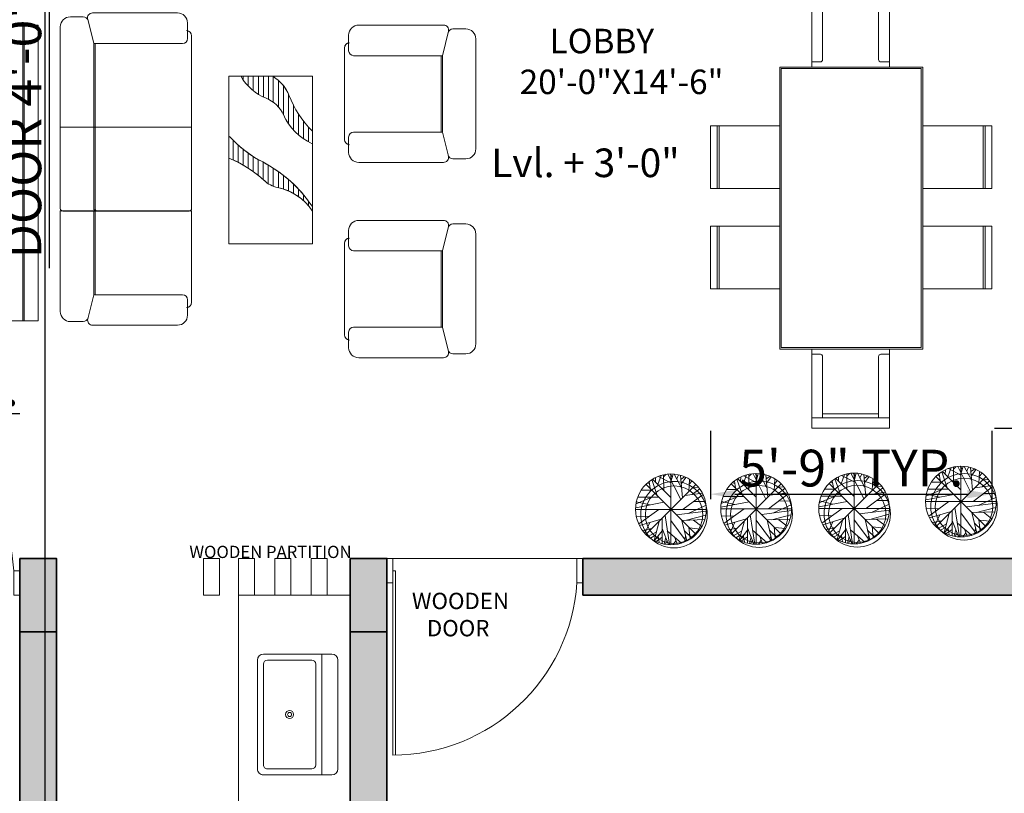
# Model space of a CAD drawing. Units: millimetres. Extents: x 595116 to 630915, y 909473 to 920225.
# Tile 120 of 134: x 629505 to 629746, y 919552 to 919742. Entities that reach past the tile are written whole.
import ezdxf

# ---------------------------------------------------------------- set-up
doc = ezdxf.new("R2010")
doc.units = ezdxf.units.MM
for name, color, linetype, lineweight in [('A-ANNO-SYMB', 7, 'Continuous', 18), ('A-AREA-IDEN', 7, 'Continuous', 20), ('A-FLOR-FIXT', 9, 'Continuous', 18), ('A-FLOR-SCRN', 31, 'Continuous', 18), ('A-FURN', 32, 'Continuous', 18), ('A-WALL', 1, 'Continuous', 35), ('A-WALL-PATT', 8, 'Continuous', 13), ('Column', 6, 'Continuous', 35), ('Dimension', 3, 'Continuous', 18), ('Doors', 31, 'Continuous', 20), ('L-PLNT', 85, 'Continuous', 13), ('Text', 7, 'Continuous', 18)]:
    doc.layers.add(name, color=color, linetype=linetype, lineweight=lineweight)
doc.styles.get("Standard").update_dxf_attribs({"font": 'arial.ttf'})
doc.dimstyles.new('ISO-25', dxfattribs={"dimtxt": 9, "dimasz": 6, "dimexe": 1.25, "dimexo": 0.625, "dimtad": 1, "dimlunit": 4, "dimtxsty": 'Standard', "dimcen": 2.5, "dimadec": 0, "dimazin": 0, "dimtfac": 1, "dimtmove": 0, "dimatfit": 3, "dimfxl": 1, "dimarcsym": 0})

# ---------------------------------------------------------------- blocks, each defined once
blk = doc.blocks.new('KWD')
for points in [[(629753.63, 919957.93), (629752.54, 919957.93), (629752.54, 919953.43), (629753.63, 919953.43)], [(629787.45, 919957.93), (629787.45, 919953.43), (629788.54, 919953.43), (629788.54, 919957.93)]]:
    blk.add_lwpolyline(points, close=True)
blk.add_lwpolyline([(629753.63, 919921.79), (629753.63, 919955.68), (629754.13, 919955.68), (629754.13, 919921.8)])
blk.add_arc((629753.64, 919955.68), 33.88, 269.99, 356.196)
blk = doc.blocks.new('DINING')
for p, q in [((630176.61, 919568.69), (630176.61, 919601.05)), ((630176.61, 919601.05), (630208.41, 919601.05)), ((630208.41, 919601.05), (630208.41, 919568.69)), ((630176.61, 919596.78), (630208.41, 919596.78)), ((630181.05, 919571.76), (630181.05, 919596.78)), ((630181.05, 919595.21), (630203.97, 919595.21)), ((630203.97, 919571.76), (630203.97, 919596.78)), ((630176.61, 919570.82), (630180.11, 919570.82)), ((630208.41, 919570.82), (630204.91, 919570.82)), ((630163.47, 919568.69), (630222.04, 919568.69)), ((630163.47, 919453.21), (630163.47, 919568.69)), ((630164.11, 919568.05), (630221.39, 919568.05)), ((630164.11, 919453.85), (630164.11, 919568.05)), ((630221.39, 919568.05), (630221.39, 919453.85)), ((630222.04, 919568.69), (630222.04, 919453.21)), ((630163.47, 919544.57), (630135.12, 919544.57)), ((630135.12, 919544.57), (630135.12, 919519)), ((630137.93, 919544.57), (630137.93, 919519)), ((630138.72, 919544.57), (630138.72, 919519)), ((630222.04, 919544.57), (630250.39, 919544.57)), ((630246.79, 919544.57), (630246.79, 919519)), ((630247.58, 919544.57), (630247.58, 919519)), ((630250.39, 919544.57), (630250.39, 919519)), ((630135.12, 919519), (630163.47, 919519)), ((630250.39, 919519), (630222.04, 919519)), ((630163.47, 919503.52), (630135.12, 919503.52)), ((630135.12, 919503.52), (630135.12, 919477.96)), ((630137.93, 919503.52), (630137.93, 919477.96)), ((630138.72, 919503.52), (630138.72, 919477.96)), ((630222.04, 919503.52), (630250.39, 919503.52)), ((630246.79, 919503.52), (630246.79, 919477.96)), ((630247.58, 919503.52), (630247.58, 919477.96)), ((630250.39, 919503.52), (630250.39, 919477.96)), ((630135.12, 919477.96), (630163.47, 919477.96)), ((630250.39, 919477.96), (630222.04, 919477.96)), ((630222.04, 919453.21), (630163.47, 919453.21)), ((630221.39, 919453.85), (630164.11, 919453.85)), ((630176.61, 919453.21), (630176.61, 919420.86)), ((630208.41, 919420.86), (630208.41, 919453.21)), ((630176.61, 919451.09), (630180.11, 919451.09)), ((630181.05, 919450.14), (630181.05, 919425.13)), ((630203.97, 919450.14), (630203.97, 919425.13)), ((630208.41, 919451.09), (630204.91, 919451.09)), ((630176.61, 919425.13), (630208.41, 919425.13)), ((630181.05, 919426.7), (630203.97, 919426.7)), ((630176.61, 919420.86), (630208.41, 919420.86))]:
    blk.add_line(p, q)
for centre, start, end in [((630180.11, 919571.76), 270, 0), ((630204.91, 919571.76), 180, 270), ((630180.11, 919450.14), 0, 90), ((630204.91, 919450.14), 90, 180)]:
    blk.add_arc(centre, 0.945, start, end)
blk = doc.blocks.new('SOFA')
for p, q in [((629520.59, 919742.63), (629517.45, 919742.63)), ((629517.45, 919742.63), (629520.59, 919742.63)), ((629521.79, 919741.7), (629521.7, 919742.06)), ((629521.7, 919742.06), (629523.2, 919736.06)), ((629543.7, 919743.59), (629522.89, 919743.59)), ((629522.89, 919743.59), (629543.7, 919743.59)), ((629514.98, 919740.17), (629514.98, 919695.65)), ((629514.98, 919695.65), (629514.98, 919740.17)), ((629546.16, 919741.12), (629546.16, 919739.22)), ((629546.16, 919741.12), (629546.16, 919737.29)), ((629588.11, 919740.62), (629608.91, 919740.62)), ((629588.11, 919740.62), (629608.91, 919740.62)), ((629611.21, 919739.66), (629614.36, 919739.66)), ((629611.21, 919739.66), (629614.36, 919739.66)), ((629547.17, 919738.01), (629547.17, 919695.65)), ((629547.17, 919738.01), (629547.17, 919695.65)), ((629585.64, 919738.15), (629585.64, 919734.33)), ((629585.64, 919736.25), (629585.64, 919738.15)), ((629610.11, 919739.09), (629608.61, 919733.09)), ((629610.11, 919739.09), (629610.02, 919738.73)), ((629616.82, 919737.2), (629616.82, 919710.3)), ((629616.82, 919737.2), (629616.82, 919710.3)), ((629523.2, 919736.06), (629523.2, 919695.65)), ((629523.2, 919695.65), (629523.2, 919736.06)), ((629523.2, 919695.65), (629523.2, 919736.06)), ((629544.93, 919736.06), (629523.2, 919736.06)), ((629523.2, 919736.06), (629523.53, 919736.06)), ((629523.2, 919736.06), (629523.53, 919736.06)), ((629523.53, 919736.06), (629523.53, 919695.65)), ((629523.53, 919736.06), (629523.53, 919695.65)), ((629523.53, 919736.06), (629523.53, 919695.65)), ((629584.64, 919735.04), (629584.64, 919712.53)), ((629584.64, 919712.53), (629584.64, 919735.04)), ((629586.87, 919733.09), (629608.61, 919733.09)), ((629608.28, 919733.09), (629608.61, 919733.09)), ((629608.28, 919714.4), (629608.28, 919733.09)), ((629608.28, 919733.09), (629608.28, 919714.4)), ((629608.61, 919733.09), (629608.61, 919714.4)), ((629608.61, 919733.09), (629608.61, 919714.4)), ((629556.25, 919728.06), (629556.25, 919687.01)), ((629556.25, 919687.01), (629556.25, 919728.06)), ((629576.77, 919728.06), (629556.25, 919728.06)), ((629556.25, 919728.06), (629576.77, 919728.06)), ((629559.82, 919728), (629559.82, 919727.13)), ((629561.06, 919728), (629561.06, 919725.63)), ((629562.29, 919728), (629562.29, 919724.5)), ((629563.52, 919728), (629563.52, 919723.63)), ((629564.75, 919728), (629564.75, 919722.96)), ((629565.98, 919728), (629565.98, 919722.42)), ((629567.19, 919727.97), (629567.19, 919721.68)), ((629576.77, 919687.01), (629576.77, 919728.06)), ((629576.77, 919728.06), (629576.77, 919687.01)), ((629568.42, 919727.08), (629568.42, 919720.54)), ((629569.65, 919725.8), (629569.65, 919718.67)), ((629569.65, 919725.8), (629569.65, 919718.67)), ((629570.88, 919723.75), (629570.88, 919716.49)), ((629570.88, 919716.49), (629570.88, 919723.75)), ((629572.12, 919720.99), (629572.12, 919714.94)), ((629573.35, 919718.86), (629573.35, 919713.74)), ((629547.17, 919715.59), (629514.98, 919715.59)), ((629574.58, 919717.12), (629574.58, 919712.78)), ((629575.81, 919715.64), (629575.81, 919712.02)), ((629585.64, 919709.42), (629585.64, 919713.17)), ((629586.87, 919714.4), (629608.61, 919714.4)), ((629608.61, 919714.4), (629608.28, 919714.4)), ((629610.09, 919708.48), (629608.61, 919714.4)), ((629557.33, 919712.4), (629557.33, 919707.56)), ((629557.33, 919707.56), (629557.33, 919712.4)), ((629558.57, 919711.23), (629558.57, 919706.97)), ((629585.64, 919709.42), (629585.64, 919711.32)), ((629559.8, 919710.18), (629559.8, 919706.31)), ((629561.03, 919709.25), (629561.03, 919705.57)), ((629562.26, 919708.41), (629562.26, 919704.73)), ((629610.02, 919708.77), (629610.09, 919708.48)), ((629563.49, 919707.66), (629563.49, 919703.8)), ((629564.72, 919706.99), (629564.72, 919702.74)), ((629565.96, 919706.31), (629565.96, 919701.75)), ((629588.11, 919706.95), (629608.89, 919706.95)), ((629608.89, 919706.95), (629588.11, 919706.95)), ((629611.21, 919707.83), (629611.48, 919707.83)), ((629611.48, 919707.83), (629611.21, 919707.83)), ((629611.48, 919707.83), (629614.36, 919707.83)), ((629614.36, 919707.83), (629611.48, 919707.83)), ((629567.19, 919705.56), (629567.19, 919701.12)), ((629568.42, 919704.73), (629568.42, 919700.78)), ((629569.65, 919703.81), (629569.65, 919700.45)), ((629570.88, 919702.8), (629570.88, 919699.98)), ((629572.12, 919701.68), (629572.12, 919699.37)), ((629573.35, 919700.43), (629573.35, 919698.59)), ((629574.58, 919699.04), (629574.58, 919697.6)), ((629575.81, 919697.48), (629575.81, 919696.34)), ((629575.81, 919697.48), (629575.81, 919696.34)), ((629547.17, 919695.06), (629514.98, 919695.06)), ((629514.98, 919695.06), (629514.98, 919670.42)), ((629514.98, 919670.42), (629514.98, 919695.06)), ((629514.98, 919695.06), (629515.44, 919695.06)), ((629515.6, 919695.04), (629546.55, 919695.04)), ((629523.2, 919695.06), (629523.2, 919674.53)), ((629523.2, 919674.53), (629523.2, 919695.04)), ((629523.2, 919674.53), (629523.2, 919695.04)), ((629523.2, 919695.04), (629523.53, 919695.04)), ((629523.2, 919695.04), (629523.53, 919695.04)), ((629523.53, 919695.04), (629523.53, 919695.11)), ((629523.53, 919695.04), (629523.53, 919695.11)), ((629523.53, 919695.06), (629523.53, 919674.53)), ((629523.53, 919695.04), (629523.53, 919674.53)), ((629523.53, 919695.04), (629523.53, 919674.53)), ((629524.14, 919695.04), (629523.53, 919695.04)), ((629524.14, 919695.04), (629523.53, 919695.04)), ((629546.71, 919695.06), (629547.17, 919695.06)), ((629547.17, 919695.06), (629547.17, 919672.66)), ((629547.17, 919695.06), (629547.17, 919672.66)), ((629588.11, 919692.76), (629608.89, 919692.76)), ((629608.89, 919692.76), (629588.11, 919692.76)), ((629611.21, 919691.88), (629611.48, 919691.88)), ((629611.48, 919691.88), (629611.21, 919691.88)), ((629611.48, 919691.88), (629614.36, 919691.88)), ((629614.36, 919691.88), (629611.48, 919691.88)), ((629585.64, 919690.3), (629585.64, 919688.39)), ((629585.64, 919690.3), (629585.64, 919686.55)), ((629610.09, 919691.23), (629608.61, 919685.31)), ((629610.02, 919690.95), (629610.09, 919691.23)), ((629616.82, 919662.52), (629616.82, 919689.42)), ((629616.82, 919662.52), (629616.82, 919689.42)), ((629556.25, 919687.01), (629576.77, 919687.01)), ((629576.77, 919687.01), (629556.25, 919687.01)), ((629584.64, 919664.68), (629584.64, 919687.18)), ((629584.64, 919687.18), (629584.64, 919664.68)), ((629586.87, 919685.31), (629608.61, 919685.31)), ((629608.61, 919685.31), (629608.28, 919685.31)), ((629608.28, 919685.31), (629608.28, 919666.62)), ((629608.28, 919666.62), (629608.28, 919685.31)), ((629608.61, 919666.62), (629608.61, 919685.31)), ((629608.61, 919666.62), (629608.61, 919685.31)), ((629521.72, 919668.61), (629523.2, 919674.53)), ((629544.93, 919674.53), (629523.2, 919674.53)), ((629523.53, 919674.53), (629523.2, 919674.53)), ((629523.53, 919674.53), (629523.2, 919674.53)), ((629546.16, 919669.54), (629546.16, 919673.3)), ((629546.16, 919671.45), (629546.16, 919669.54)), ((629520.32, 919667.96), (629517.45, 919667.96)), ((629520.32, 919667.96), (629517.45, 919667.96)), ((629520.59, 919667.96), (629520.32, 919667.96)), ((629520.59, 919667.96), (629520.32, 919667.96)), ((629521.72, 919668.61), (629521.79, 919668.89)), ((629543.7, 919667.08), (629522.91, 919667.08)), ((629543.7, 919667.08), (629522.91, 919667.08)), ((629585.64, 919661.56), (629585.64, 919665.39)), ((629586.87, 919666.62), (629608.61, 919666.62)), ((629608.28, 919666.62), (629608.61, 919666.62)), ((629610.11, 919660.63), (629608.61, 919666.62)), ((629585.64, 919663.47), (629585.64, 919661.56)), ((629610.11, 919660.63), (629610.02, 919660.99)), ((629611.21, 919660.05), (629614.36, 919660.05)), ((629611.21, 919660.05), (629614.36, 919660.05)), ((629588.11, 919659.1), (629608.91, 919659.1)), ((629588.11, 919659.1), (629608.91, 919659.1))]:
    blk.add_line(p, q)
for centre, radius, start, end in [((629517.45, 919740.17), 2.46, 90, 180), ((629517.45, 919740.17), 2.46, 90, 180), ((629520.59, 919741.4), 1.23, 14.0362, 90), ((629520.59, 919741.4), 1.23, 14.0362, 90), ((629522.89, 919742.36), 1.23, 90, 194.0362), ((629522.89, 919742.36), 1.23, 90, 194.0362), ((629543.7, 919741.12), 2.46, 0, 90), ((629543.7, 919741.12), 2.46, 0, 90), ((629588.11, 919738.15), 2.46, 90, 180), ((629588.11, 919738.15), 2.46, 90, 180), ((629608.91, 919739.39), 1.23, 345.9638, 90), ((629608.91, 919739.39), 1.23, 345.9638, 90), ((629611.21, 919738.43), 1.23, 90, 165.9638), ((629611.21, 919738.43), 1.23, 90, 165.9638), ((629614.36, 919737.2), 2.46, 0, 90), ((629614.36, 919737.2), 2.46, 0, 90), ((629544.93, 919737.29), 1.23, 270, 0), ((629545.94, 919738.01), 1.23, 0, 90), ((629545.94, 919738.01), 1.23, 0, 79.4007), ((629585.87, 919735.04), 1.23, 90, 180), ((629585.87, 919735.04), 1.23, 100.5993, 180), ((629586.87, 919734.33), 1.23, 180, 270), ((629570.11, 919734.3), 12.54, 210.2644, 248.0021), ((629562.37, 919720.03), 9.29, 21.2599, 58.8091), ((629562.37, 919720.03), 9.29, 23.6102, 38.4008), ((629562.42, 919715.26), 7.99, 24.8088, 68.0021), ((629594.57, 919732.56), 25.26, 201.2599, 225.1217), ((629582.84, 919724.7), 14.51, 204.5645, 214.4539), ((629582.84, 919724.7), 14.51, 204.8088, 245.1378), ((629577.93, 919732.79), 28.98, 222.2366, 242.5747), ((629586.87, 919713.17), 1.23, 90, 180), ((629577.93, 919732.79), 28.98, 224.7026, 242.5747), ((629585.87, 919712.53), 1.23, 180, 270), ((629585.87, 919712.53), 1.23, 180, 259.4007), ((629588.11, 919709.42), 2.46, 180, 270), ((629588.11, 919709.42), 2.46, 180, 270), ((629608.89, 919708.18), 1.23, 270, 14.0362), ((629608.89, 919708.18), 1.23, 270, 14.0362), ((629611.21, 919709.06), 1.23, 194.0362, 270), ((629611.21, 919709.06), 1.23, 194.0362, 270), ((629614.36, 919710.3), 2.46, 270, 0), ((629614.36, 919710.3), 2.46, 270, 0), ((629546.11, 919682.25), 27.68, 46.9747, 68.4773), ((629546.11, 919682.25), 27.68, 46.9747, 66.0851), ((629549.56, 919678.1), 32.63, 33.5604, 62.5747), ((629549.56, 919678.1), 32.63, 36.4252, 62.5747), ((629569.57, 919707.39), 6.7, 226.9747, 258.3827), ((629569.57, 919707.39), 6.7, 226.9746, 258.3828), ((629565.49, 919687.55), 13.55, 33.8658, 78.3827), ((629565.49, 919687.55), 13.55, 40.4201, 78.3827), ((629515.6, 919695.65), 0.616, 180, 270), ((629515.6, 919695.65), 0.616, 180, 255.079), ((629523.81, 919695.65), 0.616, 180, 270), ((629523.81, 919695.65), 0.616, 180, 242.2854), ((629523.81, 919695.65), 0.616, 180, 242.2854), ((629524.14, 919695.65), 0.616, 180, 270), ((629524.14, 919695.65), 0.616, 180, 270), ((629524.14, 919695.65), 0.616, 180, 270), ((629546.55, 919695.65), 0.616, 270, 0), ((629546.55, 919695.65), 0.616, 284.921, 0), ((629588.11, 919690.3), 2.46, 90, 180), ((629588.11, 919690.3), 2.46, 90, 180), ((629608.89, 919691.53), 1.23, 345.9638, 90), ((629608.89, 919691.53), 1.23, 345.9638, 90), ((629611.21, 919690.65), 1.23, 90, 165.9638), ((629611.21, 919690.65), 1.23, 90, 165.9638), ((629614.36, 919689.42), 2.46, 0, 90), ((629614.36, 919689.42), 2.46, 0, 90), ((629585.87, 919687.18), 1.23, 90, 180), ((629585.87, 919687.18), 1.23, 100.5993, 180), ((629586.87, 919686.55), 1.23, 180, 270), ((629544.93, 919673.3), 1.23, 0, 90), ((629545.94, 919672.66), 1.23, 270, 0), ((629545.94, 919672.66), 1.23, 280.5993, 0), ((629517.45, 919670.42), 2.46, 180, 270), ((629517.45, 919670.42), 2.46, 180, 270), ((629520.59, 919669.19), 1.23, 270, 345.9638), ((629520.59, 919669.19), 1.23, 270, 345.9638), ((629522.91, 919668.31), 1.23, 165.9638, 270), ((629522.91, 919668.31), 1.23, 165.9638, 270), ((629543.7, 919669.54), 2.46, 270, 0), ((629543.7, 919669.54), 2.46, 270, 0), ((629586.87, 919665.39), 1.23, 90, 180), ((629585.87, 919664.68), 1.23, 180, 270), ((629585.87, 919664.68), 1.23, 180, 259.4007), ((629614.36, 919662.52), 2.46, 270, 0), ((629614.36, 919662.52), 2.46, 270, 0), ((629588.11, 919661.56), 2.46, 180, 270), ((629588.11, 919661.56), 2.46, 180, 270), ((629608.91, 919660.33), 1.23, 270, 14.0362), ((629608.91, 919660.33), 1.23, 270, 14.0362), ((629611.21, 919661.28), 1.23, 194.0362, 270), ((629611.21, 919661.28), 1.23, 194.0362, 270)]:
    blk.add_arc(centre, radius, start, end)
at = {"flags": 9}
for tag in ['XSIZE', 'YSIZE']:
    blk.add_attdef(tag, (629556.25, 919728.06), '', height=0.0205, rotation=270, dxfattribs=at)
blk = doc.blocks.new('Sink-single - 30 in top')
blk.add_line((-15, -3.999996), (15, -3.999996))
for points in [[(-13.5, 0), (13.5, 0)], [(-15, -18.499996), (-15, -1.5)], [(15, -1.5), (15, -18.499996)], [(-13.5, -17.499996), (-13.5, -6.499996)], [(-12.5, -5.499996), (12.5, -5.499996)], [(13.5, -6.499996), (13.5, -17.499996)], [(12.5, -18.499996), (-12.5, -18.499996)], [(13.5, -19.999996), (-13.5, -19.999996)]]:
    blk.add_lwpolyline(points)
for radius in [1, 0.5]:
    blk.add_circle((0, -11.999996), radius)
for centre, radius, start, end in [((-13.5, -1.5), 1.5, 90, 180), ((13.5, -1.5), 1.5, 0, 90), ((-12.5, -6.499996), 1, 90, 180), ((12.5, -6.499996), 1, 0, 90), ((-13.5, -18.499996), 1.5, 180, 270), ((-12.5, -17.499996), 1, 180, 270), ((12.5, -17.499996), 1, 270, 0), ((13.5, -18.499996), 1.5, 270, 0)]:
    blk.add_arc(centre, radius, start, end)
blk = doc.blocks.new('POTTED-PLANT')
for p, q in [((4.85, 16.17), (4.88, 17.22)), ((5.49, 15.52), (6.28, 17.77)), ((5.61, 17.51), (8.67, 15.94)), ((6.86, 17.38), (7.52, 18.03)), ((6.89, 14.08), (6.86, 17.93)), ((7.9, 18.06), (11.06, 11.86)), ((9.02, 17.38), (8.46, 18.1)), ((8.67, 18.11), (8.67, 0.76)), ((8.74, 16.47), (9.2, 18.06)), ((11.32, 14.57), (9.46, 18.06)), ((10.09, 16.89), (10.53, 17.9)), ((11.52, 12.26), (11.04, 17.77)), ((11.14, 16.82), (12.03, 17.41)), ((11.24, 15.75), (12.36, 17.28)), ((14.75, 15.51), (2.6, 3.36)), ((14.75, 3.36), (2.6, 15.51)), ((2.87, 15.88), (3.4, 15.68)), ((3.32, 16.24), (3.58, 14.57)), ((3.96, 16.73), (5.31, 12.84)), ((4.16, 16.82), (8.64, 12.35)), ((13.25, 16.79), (13.05, 13.86)), ((13.17, 15.58), (13.86, 16.4)), ((13.91, 13.07), (15.74, 14.51)), ((14.04, 14.8), (15.41, 14.87)), ((4.01, 12.42), (0.12, 10.79)), ((0.57, 12.45), (5.66, 12.45)), ((1.47, 14.18), (3.93, 14.18)), ((16.53, 13.1), (11.7, 9.48)), ((12.05, 12.81), (16.38, 13.4)), ((0.04, 9.84), (6.94, 11.18)), ((0.19, 11.28), (3.48, 10.53)), ((12.92, 8.47), (17.27, 10.46)), ((14.24, 11.38), (17.09, 11.41)), ((0, 9.44), (17.35, 9.44)), ((0.22, 7.66), (3.4, 7.75)), ((0.78, 5.86), (5.74, 9.45)), ((6.53, 7.26), (6.56, 1.1)), ((7.22, 7.98), (8.31, 0.8)), ((10.02, 8.11), (17.3, 9.03)), ((12.49, 6.77), (17.19, 8.01)), ((0.98, 5.47), (6.25, 7.04)), ((3.48, 6.19), (2.31, 3.58)), ((5.79, 6.51), (4.54, 1.82)), ((8.67, 6.68), (12.41, 1.65)), ((11.37, 6.74), (12.54, 1.72)), ((11.39, 6.74), (16.97, 6.94)), ((13.07, 5.08), (13.35, 2.21)), ((13.22, 4.91), (15.85, 4.62)), ((14.19, 6.81), (16.25, 5.24)), ((3.99, 4.75), (1.72, 4.29)), ((5.1, 3.97), (3.07, 2.83)), ((4.88, 3.09), (3.65, 2.4)), ((6.56, 4.2), (4.67, 1.78)), ((6.56, 2.6), (5.05, 1.59)), ((5.56, 2.86), (5.79, 1.33)), ((6.56, 4.78), (8.11, 0.84)), ((7.45, 2.57), (7.01, 0.97)), ((7.78, 4.2), (11.26, 1.2)), ((9.53, 2.7), (10.2, 0.97)), ((11.98, 4.16), (13.78, 2.43)), ((12.26, 2.96), (12, 1.49)), ((7.75, 1.82), (7.32, 0.93)), ((9.89, 1.75), (9.23, 0.84))]:
    blk.add_line(p, q)
for centre, radius in [((8.67, 9.44), 8.67), ((9.43, 8.14), 8.14), ((9.43, 8.14), 7.03)]:
    blk.add_circle(centre, radius)
blk = doc.blocks.new('COLUMN-RECT-9X18')
h = blk.add_hatch(color=256)
h.dxf.hatch_style = 1
h.paths.add_polyline_path([(9, 18), (0, 18), (0, 0), (9, 0)])
blk.add_lwpolyline([(0, 18), (9, 18), (9, 0), (0, 0)], close=True)
blk = doc.blocks.new('*D162')
at = {"layer": 'Defpoints', "color": 0, "transparency": 16777216}
for p in [(629505.04, 919832.11), (629505.04, 919783.93), (629512.27, 919783.93)]:
    blk.add_point(p, dxfattribs=at)
at = {"layer": 'Dimension', "color": 0, "lineweight": -2, "transparency": 16777216}
for p, q in [((629505.67, 919832.11), (629513.52, 919832.11)), ((629512.27, 919826.11), (629512.27, 919789.93)), ((629505.67, 919783.93), (629513.52, 919783.93)), ((629512.27, 919783.93), (629512.27, 919681.05))]:
    blk.add_line(p, q, dxfattribs=at)
at = {"layer": 'Dimension', "color": 0, "transparency": 16777216}
for points in [[(629511.27, 919826.11), (629513.27, 919826.11), (629512.27, 919832.11)], [(629511.27, 919789.93), (629513.27, 919789.93), (629512.27, 919783.93)]]:
    blk.add_solid(points, dxfattribs=at)
at = {"layer": 'Dimension', "color": 0, "transparency": 16777216, "insert": (629506.99, 919729.49), "char_height": 9, "attachment_point": 5, "rotation": 90}
blk.add_mtext('DOOR 4\'-0" TYP.', dxfattribs=at)
blk = doc.blocks.new('*D180')
at = {"layer": 'Defpoints', "color": 0, "transparency": 16777216}
for p in [(629743.29, 919749.69), (629759.47, 919749.69), (629743.29, 919641.85)]:
    blk.add_point(p, dxfattribs=at)
at = {"layer": 'Dimension', "color": 0, "lineweight": -2, "transparency": 16777216}
for p, q in [((629759.47, 919749.69), (629759.47, 919886.8)), ((629743.92, 919749.69), (629760.72, 919749.69)), ((629759.47, 919647.85), (629759.47, 919743.69)), ((629743.92, 919641.85), (629760.72, 919641.85))]:
    blk.add_line(p, q, dxfattribs=at)
at = {"layer": 'Dimension', "color": 0, "transparency": 16777216}
for points in [[(629758.47, 919743.69), (629760.47, 919743.69), (629759.47, 919749.69)], [(629758.47, 919647.85), (629760.47, 919647.85), (629759.47, 919641.85)]]:
    blk.add_solid(points, dxfattribs=at)
at = {"layer": 'Dimension', "color": 0, "transparency": 16777216, "insert": (629754.19, 919821.24), "char_height": 9, "attachment_point": 5, "rotation": 90}
blk.add_mtext('DINING SET 9\'-0" TYP.', dxfattribs=at)
blk = doc.blocks.new('*D181')
at = {"layer": 'Defpoints', "color": 0, "transparency": 16777216}
for p in [(629674.3, 919641.85), (629743.29, 919641.85), (629743.29, 919625.68)]:
    blk.add_point(p, dxfattribs=at)
at = {"layer": 'Dimension', "color": 0, "lineweight": -2, "transparency": 16777216}
for p, q in [((629674.3, 919641.23), (629674.3, 919624.43)), ((629743.29, 919641.23), (629743.29, 919624.43)), ((629680.3, 919625.68), (629737.29, 919625.68))]:
    blk.add_line(p, q, dxfattribs=at)
at = {"layer": 'Dimension', "color": 0, "transparency": 16777216}
for points in [[(629680.3, 919626.68), (629680.3, 919624.68), (629674.3, 919625.68)], [(629737.29, 919626.68), (629737.29, 919624.68), (629743.29, 919625.68)]]:
    blk.add_solid(points, dxfattribs=at)
at = {"layer": 'Dimension', "color": 0, "transparency": 16777216, "insert": (629708.8, 919630.9), "char_height": 9, "attachment_point": 5}
blk.add_mtext('5\'-9" TYP.', dxfattribs=at)
blk = doc.blocks.new('*D189')
at = {"layer": 'Defpoints', "color": 0, "transparency": 16777216}
for p in [(629436.79, 919645.42), (629414.9, 919641.11), (629436.79, 919641.11)]:
    blk.add_point(p, dxfattribs=at)
at = {"layer": 'Dimension', "color": 0, "lineweight": -2, "transparency": 16777216}
for p, q in [((629414.9, 919641.74), (629414.9, 919646.67)), ((629436.79, 919641.74), (629436.79, 919646.67)), ((629420.9, 919645.42), (629430.79, 919645.42)), ((629436.79, 919645.42), (629505.05, 919645.42))]:
    blk.add_line(p, q, dxfattribs=at)
at = {"layer": 'Dimension', "color": 0, "transparency": 16777216}
for points in [[(629420.9, 919646.42), (629420.9, 919644.42), (629414.9, 919645.42)], [(629430.79, 919646.42), (629430.79, 919644.42), (629436.79, 919645.42)]]:
    blk.add_solid(points, dxfattribs=at)
at = {"layer": 'Dimension', "color": 0, "transparency": 16777216, "insert": (629473.92, 919650.64), "char_height": 9, "attachment_point": 5}
blk.add_mtext('1\'-10" TYP.', dxfattribs=at)
blk = doc.blocks.new('*D220')
at = {"layer": 'Defpoints', "color": 0, "transparency": 16777216}
for p in [(629824.95, 920160.76), (629511.27, 919302.01), (629824.95, 919302.01)]:
    blk.add_point(p, dxfattribs=at)
at = {"layer": 'Dimension', "color": 0, "lineweight": -2, "transparency": 16777216}
for p, q in [((629511.27, 919302.63), (629511.27, 920162.01)), ((629824.95, 919302.63), (629824.95, 920162.01)), ((629517.27, 920160.76), (629818.95, 920160.76))]:
    blk.add_line(p, q, dxfattribs=at)
at = {"layer": 'Dimension', "color": 0, "transparency": 16777216}
for points in [[(629517.27, 920161.76), (629517.27, 920159.76), (629511.27, 920160.76)], [(629818.95, 920161.76), (629818.95, 920159.76), (629824.95, 920160.76)]]:
    blk.add_solid(points, dxfattribs=at)
at = {"layer": 'Dimension', "color": 0, "transparency": 16777216, "insert": (629668.11, 920166.03), "char_height": 9, "attachment_point": 5}
blk.add_mtext('26\'-1 1/2"', dxfattribs=at)

msp = doc.modelspace()

# ---------------------------------------------------------------- hatches: boundary and pattern name
at = {"layer": 'A-FLOR-SCRN'}
h = msp.add_hatch(color=256, dxfattribs=at)
h.dxf.hatch_style = 1
h.paths.add_polyline_path([(629506.174, 919740.57), (629505.844, 919740.57), (629505.844, 919668.119), (629506.174, 919668.119)])
at = {"layer": 'A-WALL-PATT'}
h = msp.add_hatch(color=256, dxfattribs=at)
h.dxf.hatch_style = 1
h.paths.add_polyline_path([(629820.041, 919609.928), (629643.041, 919609.928), (629643.041, 919600.928), (629820.041, 919600.928)])
h = msp.add_hatch(color=256, dxfattribs=at)
h.dxf.hatch_style = 1
h.paths.add_polyline_path([(629514.041, 919591.928), (629505.041, 919591.928), (629505.041, 919429.828), (629514.041, 919429.828)])
h = msp.add_hatch(color=256, dxfattribs=at)
h.dxf.hatch_style = 1
h.paths.add_polyline_path([(629595.041, 919591.928), (629586.041, 919591.928), (629586.041, 919429.928), (629595.041, 919429.928)])

# ---------------------------------------------------------------- linework, layer by layer
at = {"layer": 'A-FLOR-FIXT'}
for p, q in [((629586.041, 919600.928), (629558.656, 919600.928)), ((629558.656, 919600.928), (629558.656, 919548.428))]:
    msp.add_line(p, q, dxfattribs=at)
at = {"layer": 'A-FLOR-SCRN'}
for p, q in [((629505.844, 919740.57), (629505.844, 919668.119)), ((629506.174, 919740.57), (629506.174, 919668.119))]:
    msp.add_line(p, q, dxfattribs=at)
for points in [[(629502.1, 919740.57), (629509.588, 919740.57), (629509.588, 919668.119), (629502.1, 919668.119)], [(629554.042, 919600.928), (629550.093, 919600.928), (629550.093, 919609.928), (629554.042, 919609.928)], [(629562.604, 919600.928), (629558.656, 919600.928), (629558.656, 919609.928), (629562.604, 919609.928)], [(629571.489, 919600.928), (629567.54, 919600.928), (629567.54, 919609.928), (629571.489, 919609.928)], [(629580.396, 919600.928), (629576.447, 919600.928), (629576.447, 919609.928), (629580.396, 919609.928)]]:
    msp.add_lwpolyline(points, close=True, dxfattribs=at)
at = {"layer": 'A-WALL'}
for p, q in [((629505.041, 919609.928), (629505.041, 919411.928)), ((629505.041, 919609.928), (629514.041, 919609.928)), ((629514.041, 919609.928), (629514.041, 919420.928)), ((629586.041, 919609.928), (629586.041, 919411.928)), ((629586.041, 919609.928), (629595.041, 919609.928)), ((629595.041, 919609.928), (629595.041, 919411.928)), ((629643.041, 919609.928), (629643.041, 919600.928)), ((629643.041, 919609.928), (629838.041, 919609.928)), ((629643.041, 919600.928), (629838.041, 919600.928))]:
    msp.add_line(p, q, dxfattribs=at)
at = {"layer": 'Doors'}
msp.add_line((629596.498, 919609.928), (629641.583, 919609.928), dxfattribs=at)

# ---------------------------------------------------------------- block references
at = {"layer": 'A-FLOR-FIXT', "xscale": 0.9872623020467125, "yscale": 0.9872623020467125, "zscale": 0.9872623020467125, "rotation": 270}
msp.add_blockref('Sink-single - 30 in top', (629583.022, 919571.697), dxfattribs=at)
at = {"layer": 'A-FURN', "xscale": 0.5984731567659999, "yscale": 0.5984731567659999, "zscale": 0.5984731567659999}
msp.add_blockref('DINING', (252555.352, 369393.149), dxfattribs=at)
at = {"layer": 'A-FURN'}
msp.add_blockref('SOFA', (0, 0), dxfattribs=at)
at = {"layer": 'Column'}
for p in [(629505.041, 919591.928), (629586.041, 919591.928)]:
    msp.add_blockref('COLUMN-RECT-9X18', p, dxfattribs=at)
at = {"layer": 'Doors', "xscale": -1.333333333333333, "yscale": 1.333333333333333, "zscale": 1.333333333333333, "rotation": 180}
msp.add_blockref('KWD', (-210213.014, 2146211.498), dxfattribs=at)
at = {"layer": 'Doors', "xscale": 1.333333333333333, "yscale": 1.333333333333333, "zscale": 1.333333333333333}
msp.add_blockref('KWD', (-210075.014, -307000.643), dxfattribs=at)
at = {"layer": 'L-PLNT'}
for p in [(629727.004, 919614.429), (629655.952, 919612.51), (629676.836, 919612.62), (629700.84, 919612.73)]:
    msp.add_blockref('POTTED-PLANT', p, dxfattribs=at)

# ---------------------------------------------------------------- texts
at = {"layer": 'A-ANNO-SYMB', "insert": (629607.73, 919710.358), "char_height": 7, "attachment_point": 1}
msp.add_mtext_dynamic_manual_height_columns('{      Lvl. + 3\'-0"}', width=83.57324, gutter_width=12.5, heights=[0], dxfattribs=at)
at = {"layer": 'A-AREA-IDEN', "insert": (629623.884, 919739.702), "char_height": 6, "attachment_point": 1}
msp.add_mtext_dynamic_manual_height_columns('{      LOBBY\\P  20\'-0"X14\'-6"}', width=83.57324, gutter_width=12.5, heights=[0], dxfattribs=at)
at = {"layer": 'Text', "attachment_point": 1}
for s, insert, char_height in [('{ WOODEN PARTITION}', (629545.703, 919613.032), 3), ('{     WOODEN\\P        DOOR}', (629595.041, 919601.518), 4)]:
    msp.add_mtext_dynamic_manual_height_columns(s, width=61.33456, gutter_width=12.5, heights=[0], dxfattribs=dict(at, insert=insert, char_height=char_height))

# ---------------------------------------------------------------- dimensions: what is measured, and where the dimension line sits
at = {"layer": 'Dimension'}
dim = msp.add_linear_dim(base=(629824.951, 920160.756), p1=(629511.274, 919302.009), p2=(629824.951, 919302.009), dimstyle='ISO-25', override={"dimdec": 1, "dimlfac": 1, "dimrnd": 0, "dimzin": 1, "dimdsep": 46, "dimlunit": 4, "dimfrac": 2}, dxfattribs=at)
dim.commit()
dim.dimension.update_dxf_attribs({"geometry": '*D220', "text_midpoint": (629668.113, 920166.035)})
for base, p1, p2, angle, text, picture, middle in [((629759.47, 919749.69), (629743.294, 919641.853), (629743.294, 919749.69), 90, 'DINING SET <> TYP.', '*D180', (629754.191, 919821.242)), ((629512.268, 919783.928), (629505.041, 919832.112), (629505.041, 919783.928), 270, 'DOOR <> TYP.', '*D162', (629506.987, 919729.491))]:
    dim = msp.add_linear_dim(base=base, p1=p1, p2=p2, angle=angle, text=text, dimstyle='ISO-25', override={"dimdec": 1, "dimlfac": 1, "dimrnd": 0, "dimzin": 1, "dimdsep": 46, "dimlunit": 4, "dimfrac": 2}, dxfattribs=at)
    dim.commit()
    dim.dimension.update_dxf_attribs({"geometry": picture, "text_midpoint": middle})
for base, p1, p2, picture, middle in [((629436.791, 919645.418), (629414.899, 919641.114), (629436.791, 919641.114), '*D189', (629473.918, 919650.638)), ((629743.294, 919625.677), (629674.304, 919641.853), (629743.294, 919641.853), '*D181', (629708.799, 919630.897))]:
    dim = msp.add_linear_dim(base=base, p1=p1, p2=p2, text='<> TYP.', dimstyle='ISO-25', override={"dimdec": 1, "dimlfac": 1, "dimrnd": 0, "dimzin": 1, "dimdsep": 46, "dimlunit": 4, "dimfrac": 2}, dxfattribs=at)
    dim.commit()
    dim.dimension.update_dxf_attribs({"geometry": picture, "text_midpoint": middle})

doc.saveas('drawing.dxf')
